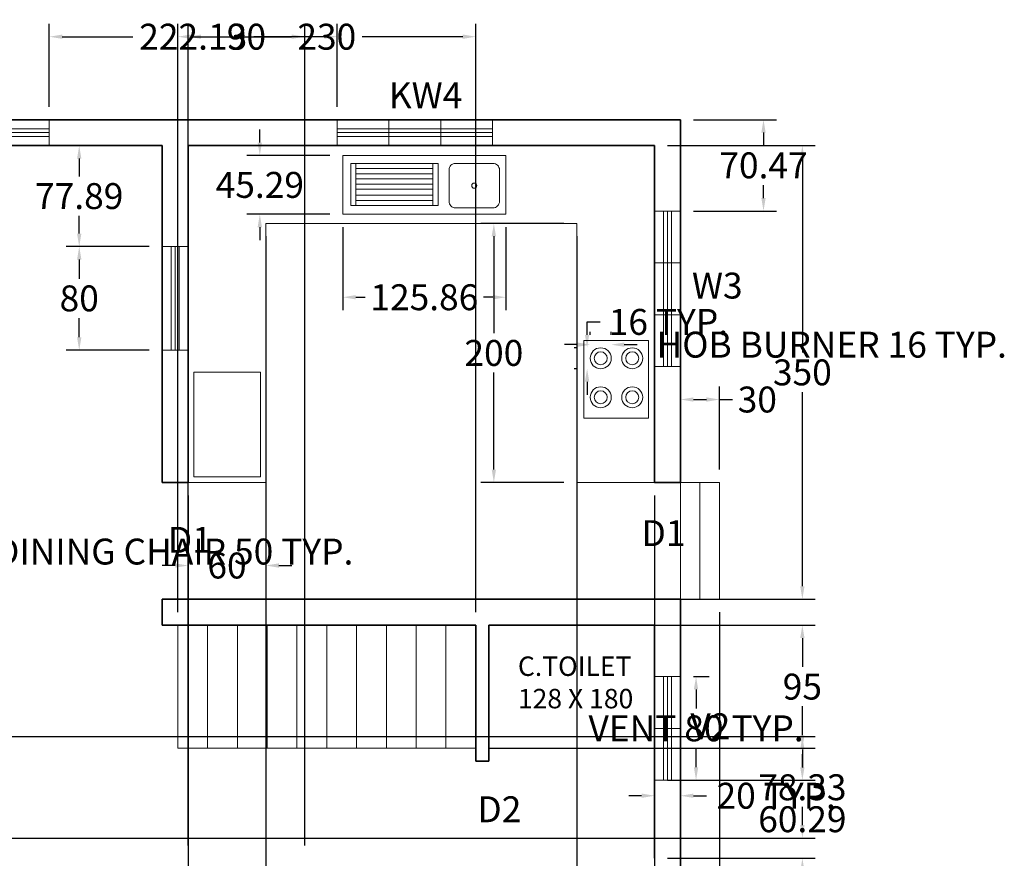
# Model space of a CAD drawing. Units: centimetres. Extents: x 543 to 2148, y 348 to 1642.
# Tile 4 of 4: x 1302 to 2062, y 995 to 1642. Entities that reach past the tile are written whole.
import ezdxf

# ---------------------------------------------------------------- set-up
doc = ezdxf.new("R2010")
doc.units = ezdxf.units.CM
doc.header["$MEASUREMENT"] = 0
for name, color, linetype, lineweight in [('A-ANNO-DIMS', 2, 'Continuous', 18), ('A-ANNO-TEXT', 7, 'Continuous', 18), ('A-AREA-IDEN', 7, 'Continuous', 25), ('A-EQPM', 9, 'Continuous', 18), ('A-FLOR-CASE', 8, 'Continuous', 20), ('A-FLOR-FIXT', 8, 'Continuous', 18), ('A-FLOR-STRS', 7, 'Continuous', 20), ('A-GLAZ', 4, 'Continuous', 18), ('A-WALL', 7, 'Continuous', 35)]:
    doc.layers.add(name, color=color, linetype=linetype, lineweight=lineweight)
doc.styles.get("Standard").update_dxf_attribs({"font": 'arial.ttf'})
doc.dimstyles.get("Standard").update_dxf_attribs({"dimtxt": 20, "dimasz": 10, "dimexe": 10, "dimexo": 10, "dimgap": 5, "dimtad": 0, "dimtih": 1, "dimtoh": 1, "dimdec": 0, "dimzin": 0, "dimdsep": 46, "dimtxsty": 'Standard', "dimcen": 5, "dimadec": 0, "dimazin": 0, "dimtfac": 1, "dimtdec": 0, "dimtofl": 0, "dimtmove": 0, "dimatfit": 3, "dimfxl": 1, "dimtolj": 1, "dimtzin": 0, "dimarcsym": 0})

# ---------------------------------------------------------------- blocks, each defined once
blk = doc.blocks.new('WIN-1200')
for p, q in [((40, 20), (40, 0)), ((80, 20), (80, 0)), ((0, 13), (120, 13)), ((0, 10), (120, 10)), ((0, 7), (120, 7))]:
    blk.add_line(p, q)
blk.add_lwpolyline([(0, 20), (120, 20), (120, 0), (0, 0)], close=True)
blk = doc.blocks.new('VENT-800')
for p, q in [((7, 80), (7, 0)), ((10, 80), (10, 0)), ((13, 80), (13, 0)), ((20, 40), (0, 40)), ((20, 0), (0, 0))]:
    blk.add_line(p, q)
blk.add_lwpolyline([(0, 0), (0, 80), (20, 80), (20, 0)])
blk = doc.blocks.new('HOB-BURNER')
for radius in [8.09, 5]:
    blk.add_circle((8.09, 8.09), radius)
blk = doc.blocks.new('*D15')
at = {"layer": 'A-ANNO-DIMS', "color": 0, "lineweight": -2, "transparency": 16777216}
for p, q in [((1218.09, 1231.81), (1248.09, 1231.81)), ((1258.09, 1231.81), (1268.09, 1231.81)), ((1208.09, 1229.31), (1208.09, 1221.81)), ((1258.09, 1229.31), (1258.09, 1221.81))]:
    blk.add_line(p, q, dxfattribs=at)
at = {"layer": 'A-ANNO-DIMS', "color": 0, "transparency": 16777216}
for points in [[(1218.09, 1233.48), (1218.09, 1230.15), (1208.09, 1231.81)], [(1248.09, 1233.48), (1248.09, 1230.15), (1258.09, 1231.81)]]:
    blk.add_solid(points, dxfattribs=at)
at = {"layer": 'Defpoints', "color": 0, "transparency": 16777216}
for p in [(1208.09, 1239.31), (1258.09, 1239.31), (1258.09, 1231.81)]:
    blk.add_point(p, dxfattribs=at)
at = {"layer": 'A-ANNO-DIMS', "color": 0, "transparency": 16777216, "insert": (1421.4, 1231.81), "char_height": 20, "attachment_point": 5}
blk.add_mtext('\\A1;DINING CHAIR 50 TYP.', dxfattribs=at)
blk = doc.blocks.new('*D17')
at = {"layer": 'A-ANNO-DIMS', "color": 0, "lineweight": -2, "transparency": 16777216}
for p, q in [((1305.14, 955.09), (1305.14, 965.09)), ((1305.14, 965.09), (1315.14, 965.09)), ((1312.14, 945.09), (1315.14, 945.09)), ((1312.14, 925.09), (1315.14, 925.09)), ((1305.14, 915.09), (1305.14, 905.09))]:
    blk.add_line(p, q, dxfattribs=at)
at = {"layer": 'A-ANNO-DIMS', "color": 0, "transparency": 16777216}
for points in [[(1303.47, 955.09), (1306.81, 955.09), (1305.14, 945.09)], [(1303.47, 915.09), (1306.81, 915.09), (1305.14, 925.09)]]:
    blk.add_solid(points, dxfattribs=at)
at = {"layer": 'Defpoints', "color": 0, "transparency": 16777216}
for p in [(1302.14, 945.09), (1305.14, 945.09), (1302.14, 925.09)]:
    blk.add_point(p, dxfattribs=at)
at = {"layer": 'A-ANNO-DIMS', "color": 0, "transparency": 16777216, "insert": (1472.79, 965.09), "char_height": 20, "attachment_point": 5}
blk.add_mtext('\\A1;SCREEN POST 20 TYP.', dxfattribs=at)
blk = doc.blocks.new('*D19')
at = {"layer": 'A-ANNO-DIMS', "color": 0, "lineweight": -2, "transparency": 16777216}
for p, q in [((1742.49, 1399.05), (1742.49, 1401.48)), ((1758.67, 1399.05), (1758.67, 1401.48)), ((1732.49, 1391.48), (1722.49, 1391.48)), ((1768.67, 1391.48), (1778.67, 1391.48))]:
    blk.add_line(p, q, dxfattribs=at)
at = {"layer": 'A-ANNO-DIMS', "color": 0, "transparency": 16777216}
for points in [[(1732.49, 1393.15), (1732.49, 1389.82), (1742.49, 1391.48)], [(1768.67, 1393.15), (1768.67, 1389.82), (1758.67, 1391.48)]]:
    blk.add_solid(points, dxfattribs=at)
at = {"layer": 'Defpoints', "color": 0, "transparency": 16777216}
for p in [(1758.67, 1391.48), (1742.49, 1389.05), (1758.67, 1389.05)]:
    blk.add_point(p, dxfattribs=at)
at = {"layer": 'A-ANNO-DIMS', "color": 0, "transparency": 16777216, "insert": (1928.84, 1391.48), "char_height": 20, "attachment_point": 5}
blk.add_mtext('\\A1;HOB BURNER 16 TYP.', dxfattribs=at)
blk = doc.blocks.new('*D20')
at = {"layer": 'A-ANNO-DIMS', "color": 0, "lineweight": -2, "transparency": 16777216}
for p, q in [((1740.06, 1399.05), (1740.06, 1409.05)), ((1740.06, 1409.05), (1750.06, 1409.05)), ((1732.49, 1389.05), (1730.06, 1389.05)), ((1732.49, 1372.87), (1730.06, 1372.87)), ((1740.06, 1362.87), (1740.06, 1352.87))]:
    blk.add_line(p, q, dxfattribs=at)
at = {"layer": 'A-ANNO-DIMS', "color": 0, "transparency": 16777216}
for points in [[(1738.39, 1399.05), (1741.73, 1399.05), (1740.06, 1389.05)], [(1738.39, 1362.87), (1741.73, 1362.87), (1740.06, 1372.87)]]:
    blk.add_solid(points, dxfattribs=at)
at = {"layer": 'Defpoints', "color": 0, "transparency": 16777216}
for p in [(1740.06, 1389.05), (1742.49, 1389.05), (1742.49, 1372.87)]:
    blk.add_point(p, dxfattribs=at)
at = {"layer": 'A-ANNO-DIMS', "color": 0, "transparency": 16777216, "insert": (1802.79, 1409.05), "char_height": 20, "attachment_point": 5}
blk.add_mtext('\\A1;16 TYP.', dxfattribs=at)
blk = doc.blocks.new('*D27')
at = {"layer": 'A-ANNO-DIMS', "color": 0, "lineweight": -2, "transparency": 16777216}
for p, q in [((1822.14, 1135.38), (1834.14, 1135.38)), ((1824.14, 1125.38), (1824.14, 1110.59)), ((1824.14, 1065.38), (1824.14, 1080.17)), ((1822.14, 1055.38), (1834.14, 1055.38))]:
    blk.add_line(p, q, dxfattribs=at)
at = {"layer": 'A-ANNO-DIMS', "color": 0, "transparency": 16777216}
for points in [[(1822.47, 1125.38), (1825.81, 1125.38), (1824.14, 1135.38)], [(1822.47, 1065.38), (1825.81, 1065.38), (1824.14, 1055.38)]]:
    blk.add_solid(points, dxfattribs=at)
at = {"layer": 'Defpoints', "color": 0, "transparency": 16777216}
for p in [(1812.14, 1135.38), (1824.14, 1135.38), (1812.14, 1055.38)]:
    blk.add_point(p, dxfattribs=at)
at = {"layer": 'A-ANNO-DIMS', "color": 0, "transparency": 16777216, "insert": (1824.14, 1095.38), "char_height": 20, "attachment_point": 5}
blk.add_mtext('\\A1;VENT 80 TYP.', dxfattribs=at)
blk = doc.blocks.new('*D28')
at = {"layer": 'A-ANNO-DIMS', "color": 0, "lineweight": -2, "transparency": 16777216}
for p, q in [((1782.14, 1043.38), (1772.14, 1043.38)), ((1792.14, 1045.38), (1792.14, 1033.38)), ((1812.14, 1045.38), (1812.14, 1033.38)), ((1822.14, 1043.38), (1832.14, 1043.38))]:
    blk.add_line(p, q, dxfattribs=at)
at = {"layer": 'A-ANNO-DIMS', "color": 0, "transparency": 16777216}
for points in [[(1782.14, 1045.05), (1782.14, 1041.72), (1792.14, 1043.38)], [(1822.14, 1045.05), (1822.14, 1041.72), (1812.14, 1043.38)]]:
    blk.add_solid(points, dxfattribs=at)
at = {"layer": 'Defpoints', "color": 0, "transparency": 16777216}
for p in [(1792.14, 1055.38), (1812.14, 1055.38), (1812.14, 1043.38)]:
    blk.add_point(p, dxfattribs=at)
at = {"layer": 'A-ANNO-DIMS', "color": 0, "transparency": 16777216, "insert": (1885.99, 1043.38), "char_height": 20, "attachment_point": 5}
blk.add_mtext('\\A1;20 TYP.', dxfattribs=at)
blk = doc.blocks.new('*D38')
at = {"layer": 'A-ANNO-DIMS', "color": 0, "lineweight": -2, "transparency": 16777216}
for p, q in [((1812.14, 1295.09), (1812.14, 1359.14)), ((1842.14, 1295.09), (1842.14, 1359.14)), ((1822.14, 1349.14), (1832.14, 1349.14)), ((1842.14, 1349.14), (1852.14, 1349.14))]:
    blk.add_line(p, q, dxfattribs=at)
at = {"layer": 'A-ANNO-DIMS', "color": 0, "transparency": 16777216}
for points in [[(1822.14, 1350.81), (1822.14, 1347.48), (1812.14, 1349.14)], [(1832.14, 1350.81), (1832.14, 1347.48), (1842.14, 1349.14)]]:
    blk.add_solid(points, dxfattribs=at)
at = {"layer": 'Defpoints', "color": 0, "transparency": 16777216}
for p in [(1842.14, 1349.14), (1812.14, 1285.09), (1842.14, 1285.09)]:
    blk.add_point(p, dxfattribs=at)
at = {"layer": 'A-ANNO-DIMS', "color": 0, "transparency": 16777216, "insert": (1871.42, 1349.14), "char_height": 20, "attachment_point": 5}
blk.add_mtext('\\A1;30', dxfattribs=at)
blk = doc.blocks.new('*D39')
at = {"layer": 'A-ANNO-DIMS', "color": 0, "lineweight": -2, "transparency": 16777216}
for p, q in [((1432.14, 1275.09), (1432.14, 351.04)), ((1792.14, 1275.09), (1792.14, 351.04)), ((1442.14, 361.04), (1585.09, 361.04)), ((1782.14, 361.04), (1639.19, 361.04))]:
    blk.add_line(p, q, dxfattribs=at)
at = {"layer": 'A-ANNO-DIMS', "color": 0, "transparency": 16777216}
for points in [[(1442.14, 362.71), (1442.14, 359.38), (1432.14, 361.04)], [(1782.14, 362.71), (1782.14, 359.38), (1792.14, 361.04)]]:
    blk.add_solid(points, dxfattribs=at)
at = {"layer": 'Defpoints', "color": 0, "transparency": 16777216}
for p in [(1432.14, 1285.09), (1792.14, 1285.09), (1792.14, 361.04)]:
    blk.add_point(p, dxfattribs=at)
at = {"layer": 'A-ANNO-DIMS', "color": 0, "transparency": 16777216, "insert": (1612.14, 361.04), "char_height": 20, "attachment_point": 5}
blk.add_mtext('\\A1;360', dxfattribs=at)
blk = doc.blocks.new('*D40')
at = {"layer": 'A-ANNO-DIMS', "color": 0, "lineweight": -2, "transparency": 16777216}
for p, q in [((1802.14, 1545.09), (1916.19, 1545.09)), ((1906.19, 1535.09), (1906.19, 1385.31)), ((1906.19, 1205.09), (1906.19, 1354.87)), ((1802.14, 1195.09), (1916.19, 1195.09))]:
    blk.add_line(p, q, dxfattribs=at)
at = {"layer": 'A-ANNO-DIMS', "color": 0, "transparency": 16777216}
for points in [[(1904.52, 1535.09), (1907.86, 1535.09), (1906.19, 1545.09)], [(1904.52, 1205.09), (1907.86, 1205.09), (1906.19, 1195.09)]]:
    blk.add_solid(points, dxfattribs=at)
at = {"layer": 'Defpoints', "color": 0, "transparency": 16777216}
for p in [(1792.14, 1545.09), (1906.19, 1545.09), (1792.14, 1195.09)]:
    blk.add_point(p, dxfattribs=at)
at = {"layer": 'A-ANNO-DIMS', "color": 0, "transparency": 16777216, "insert": (1906.19, 1370.09), "char_height": 20, "attachment_point": 5}
blk.add_mtext('\\A1;350', dxfattribs=at)
blk = doc.blocks.new('*D41')
at = {"layer": 'A-ANNO-DIMS', "color": 0, "lineweight": -2, "transparency": 16777216}
for p, q in [((1424.14, 1185.09), (1424.14, 1639.14)), ((1654.14, 1185.09), (1654.14, 1639.14)), ((1434.14, 1629.14), (1511.91, 1629.14)), ((1644.14, 1629.14), (1566.37, 1629.14))]:
    blk.add_line(p, q, dxfattribs=at)
at = {"layer": 'A-ANNO-DIMS', "color": 0, "transparency": 16777216}
for points in [[(1434.14, 1630.81), (1434.14, 1627.48), (1424.14, 1629.14)], [(1644.14, 1630.81), (1644.14, 1627.48), (1654.14, 1629.14)]]:
    blk.add_solid(points, dxfattribs=at)
at = {"layer": 'Defpoints', "color": 0, "transparency": 16777216}
for p in [(1654.14, 1629.14), (1424.14, 1175.09), (1654.14, 1175.09)]:
    blk.add_point(p, dxfattribs=at)
at = {"layer": 'A-ANNO-DIMS', "color": 0, "transparency": 16777216, "insert": (1539.14, 1629.14), "char_height": 20, "attachment_point": 5}
blk.add_mtext('\\A1;230', dxfattribs=at)
blk = doc.blocks.new('*D42')
at = {"layer": 'A-ANNO-DIMS', "color": 0, "lineweight": -2, "transparency": 16777216}
for p, q in [((1664.14, 1175.09), (1916.19, 1175.09)), ((1906.19, 1165.09), (1906.19, 1142.8)), ((1906.19, 1090.09), (1906.19, 1112.38)), ((1664.14, 1080.09), (1916.19, 1080.09))]:
    blk.add_line(p, q, dxfattribs=at)
at = {"layer": 'A-ANNO-DIMS', "color": 0, "transparency": 16777216}
for points in [[(1904.52, 1165.09), (1907.86, 1165.09), (1906.19, 1175.09)], [(1904.52, 1090.09), (1907.86, 1090.09), (1906.19, 1080.09)]]:
    blk.add_solid(points, dxfattribs=at)
at = {"layer": 'Defpoints', "color": 0, "transparency": 16777216}
for p in [(1654.14, 1175.09), (1906.19, 1175.09), (1654.14, 1080.09)]:
    blk.add_point(p, dxfattribs=at)
at = {"layer": 'A-ANNO-DIMS', "color": 0, "transparency": 16777216, "insert": (1906.19, 1127.59), "char_height": 20, "attachment_point": 5}
blk.add_mtext('\\A1;95', dxfattribs=at)
blk = doc.blocks.new('*D43')
at = {"layer": 'A-ANNO-DIMS', "color": 0, "lineweight": -2, "transparency": 16777216}
for p, q in [((1432.14, 1005.09), (1432.14, 1639.14)), ((1522.14, 1005.09), (1522.14, 1639.14)), ((1442.14, 1629.14), (1457.85, 1629.14)), ((1512.14, 1629.14), (1496.43, 1629.14))]:
    blk.add_line(p, q, dxfattribs=at)
at = {"layer": 'A-ANNO-DIMS', "color": 0, "transparency": 16777216}
for points in [[(1442.14, 1630.81), (1442.14, 1627.48), (1432.14, 1629.14)], [(1512.14, 1630.81), (1512.14, 1627.48), (1522.14, 1629.14)]]:
    blk.add_solid(points, dxfattribs=at)
at = {"layer": 'Defpoints', "color": 0, "transparency": 16777216}
for p in [(1522.14, 1629.14), (1432.14, 995.09), (1522.14, 995.09)]:
    blk.add_point(p, dxfattribs=at)
at = {"layer": 'A-ANNO-DIMS', "color": 0, "transparency": 16777216, "insert": (1477.14, 1629.14), "char_height": 20, "attachment_point": 5}
blk.add_mtext('\\A1;90', dxfattribs=at)
blk = doc.blocks.new('*D50')
at = {"layer": 'A-ANNO-DIMS', "color": 0, "lineweight": -2, "transparency": 16777216}
for p, q in [((1325.01, 1575.09), (1325.01, 1639.14)), ((1547.14, 1575.09), (1547.14, 1639.14)), ((1335.01, 1629.14), (1389.39, 1629.14)), ((1537.14, 1629.14), (1482.76, 1629.14))]:
    blk.add_line(p, q, dxfattribs=at)
at = {"layer": 'A-ANNO-DIMS', "color": 0, "transparency": 16777216}
for points in [[(1335.01, 1630.81), (1335.01, 1627.48), (1325.01, 1629.14)], [(1537.14, 1630.81), (1537.14, 1627.48), (1547.14, 1629.14)]]:
    blk.add_solid(points, dxfattribs=at)
at = {"layer": 'Defpoints', "color": 0, "transparency": 16777216}
for p in [(1547.14, 1629.14), (1325.01, 1565.09), (1547.14, 1565.09)]:
    blk.add_point(p, dxfattribs=at)
at = {"layer": 'A-ANNO-DIMS', "color": 0, "transparency": 16777216, "insert": (1436.07, 1629.14), "char_height": 20, "attachment_point": 5}
blk.add_mtext('\\A1;222.13', dxfattribs=at)
blk = doc.blocks.new('*D51')
at = {"layer": 'A-ANNO-DIMS', "color": 0, "lineweight": -2, "transparency": 16777216}
for p, q in [((1822.14, 1565.09), (1886.19, 1565.09)), ((1876.19, 1555.09), (1876.19, 1545.07)), ((1876.19, 1504.62), (1876.19, 1514.64)), ((1822.14, 1494.62), (1886.19, 1494.62))]:
    blk.add_line(p, q, dxfattribs=at)
at = {"layer": 'A-ANNO-DIMS', "color": 0, "transparency": 16777216}
for points in [[(1874.52, 1555.09), (1877.86, 1555.09), (1876.19, 1565.09)], [(1874.52, 1504.62), (1877.86, 1504.62), (1876.19, 1494.62)]]:
    blk.add_solid(points, dxfattribs=at)
at = {"layer": 'Defpoints', "color": 0, "transparency": 16777216}
for p in [(1812.14, 1565.09), (1812.14, 1494.62), (1876.19, 1494.62)]:
    blk.add_point(p, dxfattribs=at)
at = {"layer": 'A-ANNO-DIMS', "color": 0, "transparency": 16777216, "insert": (1876.19, 1529.85), "char_height": 20, "attachment_point": 5}
blk.add_mtext('\\A1;70.47', dxfattribs=at)
blk = doc.blocks.new('*D52')
at = {"layer": 'A-ANNO-DIMS', "color": 0, "lineweight": -2, "transparency": 16777216}
for p, q in [((1906.19, 1065.38), (1906.19, 1075.38)), ((1802.14, 1055.38), (1916.19, 1055.38)), ((1802.14, 995.09), (1916.19, 995.09)), ((1906.19, 985.09), (1906.19, 975.09))]:
    blk.add_line(p, q, dxfattribs=at)
at = {"layer": 'A-ANNO-DIMS', "color": 0, "transparency": 16777216}
for points in [[(1904.52, 1065.38), (1907.86, 1065.38), (1906.19, 1055.38)], [(1904.52, 985.09), (1907.86, 985.09), (1906.19, 995.09)]]:
    blk.add_solid(points, dxfattribs=at)
at = {"layer": 'Defpoints', "color": 0, "transparency": 16777216}
for p in [(1792.14, 1055.38), (1906.19, 1055.38), (1792.14, 995.09)]:
    blk.add_point(p, dxfattribs=at)
at = {"layer": 'A-ANNO-DIMS', "color": 0, "transparency": 16777216, "insert": (1906.19, 1025.24), "char_height": 20, "attachment_point": 5}
blk.add_mtext('\\A1;60.29', dxfattribs=at)
blk = doc.blocks.new('*D59')
at = {"layer": 'A-ANNO-DIMS', "color": 0, "lineweight": -2, "transparency": 16777216}
for p, q in [((717.14, 1089.08), (1916.19, 1089.08)), ((1906.19, 1079.08), (1906.19, 1065.14)), ((1906.19, 1020.76), (1906.19, 1034.7)), ((717.14, 1010.76), (1916.19, 1010.76))]:
    blk.add_line(p, q, dxfattribs=at)
at = {"layer": 'A-ANNO-DIMS', "color": 0, "transparency": 16777216}
for points in [[(1904.52, 1079.08), (1907.86, 1079.08), (1906.19, 1089.08)], [(1904.52, 1020.76), (1907.86, 1020.76), (1906.19, 1010.76)]]:
    blk.add_solid(points, dxfattribs=at)
at = {"layer": 'Defpoints', "color": 0, "transparency": 16777216}
for p in [(707.14, 1089.08), (1906.19, 1089.08), (707.14, 1010.76)]:
    blk.add_point(p, dxfattribs=at)
at = {"layer": 'A-ANNO-DIMS', "color": 0, "transparency": 16777216, "insert": (1906.19, 1049.92), "char_height": 20, "attachment_point": 5}
blk.add_mtext('\\A1;78.33', dxfattribs=at)
blk = doc.blocks.new('*D61')
at = {"layer": 'A-ANNO-DIMS', "color": 0, "lineweight": -2, "transparency": 16777216}
for p, q in [((1492.14, 1475.09), (1492.14, 351.04)), ((1732.14, 1475.09), (1732.14, 351.04)), ((1502.14, 361.04), (1584.91, 361.04)), ((1722.14, 361.04), (1639.37, 361.04))]:
    blk.add_line(p, q, dxfattribs=at)
at = {"layer": 'A-ANNO-DIMS', "color": 0, "transparency": 16777216}
for points in [[(1502.14, 362.71), (1502.14, 359.38), (1492.14, 361.04)], [(1722.14, 362.71), (1722.14, 359.38), (1732.14, 361.04)]]:
    blk.add_solid(points, dxfattribs=at)
at = {"layer": 'Defpoints', "color": 0, "transparency": 16777216}
for p in [(1492.14, 1485.09), (1732.14, 1485.09), (1732.14, 361.04)]:
    blk.add_point(p, dxfattribs=at)
at = {"layer": 'A-ANNO-DIMS', "color": 0, "transparency": 16777216, "insert": (1612.14, 361.04), "char_height": 20, "attachment_point": 5}
blk.add_mtext('\\A1;240', dxfattribs=at)
blk = doc.blocks.new('*D62')
at = {"layer": 'A-ANNO-DIMS', "color": 0, "lineweight": -2, "transparency": 16777216}
for p, q in [((1722.14, 1485.09), (1658.09, 1485.09)), ((1668.09, 1475.09), (1668.09, 1400.3)), ((1668.09, 1295.09), (1668.09, 1369.88)), ((1722.14, 1285.09), (1658.09, 1285.09))]:
    blk.add_line(p, q, dxfattribs=at)
at = {"layer": 'A-ANNO-DIMS', "color": 0, "transparency": 16777216}
for points in [[(1666.42, 1475.09), (1669.76, 1475.09), (1668.09, 1485.09)], [(1666.42, 1295.09), (1669.76, 1295.09), (1668.09, 1285.09)]]:
    blk.add_solid(points, dxfattribs=at)
at = {"layer": 'Defpoints', "color": 0, "transparency": 16777216}
for p in [(1668.09, 1485.09), (1732.14, 1485.09), (1732.14, 1285.09)]:
    blk.add_point(p, dxfattribs=at)
at = {"layer": 'A-ANNO-DIMS', "color": 0, "transparency": 16777216, "insert": (1668.09, 1385.09), "char_height": 20, "attachment_point": 5}
blk.add_mtext('\\A1;200', dxfattribs=at)
blk = doc.blocks.new('*D63')
at = {"layer": 'A-ANNO-DIMS', "color": 0, "lineweight": -2, "transparency": 16777216}
for p, q in [((1432.14, 1275.09), (1432.14, 1211.04)), ((1492.14, 1275.09), (1492.14, 1211.04)), ((1422.14, 1221.04), (1412.14, 1221.04)), ((1502.14, 1221.04), (1512.14, 1221.04))]:
    blk.add_line(p, q, dxfattribs=at)
at = {"layer": 'A-ANNO-DIMS', "color": 0, "transparency": 16777216}
for points in [[(1422.14, 1222.71), (1422.14, 1219.38), (1432.14, 1221.04)], [(1502.14, 1222.71), (1502.14, 1219.38), (1492.14, 1221.04)]]:
    blk.add_solid(points, dxfattribs=at)
at = {"layer": 'Defpoints', "color": 0, "transparency": 16777216}
for p in [(1432.14, 1285.09), (1492.14, 1285.09), (1432.14, 1221.04)]:
    blk.add_point(p, dxfattribs=at)
at = {"layer": 'A-ANNO-DIMS', "color": 0, "transparency": 16777216, "insert": (1462.14, 1221.04), "char_height": 20, "attachment_point": 5}
blk.add_mtext('\\A1;60', dxfattribs=at)
blk = doc.blocks.new('*D68')
at = {"layer": 'A-ANNO-DIMS', "color": 0, "lineweight": -2, "transparency": 16777216}
for p, q in [((1842.14, 1185.09), (1842.14, 351.04)), ((637.14, 415.09), (637.14, 351.04)), ((647.14, 361.04), (1205.64, 361.04)), ((1832.14, 361.04), (1273.64, 361.04))]:
    blk.add_line(p, q, dxfattribs=at)
at = {"layer": 'A-ANNO-DIMS', "color": 0, "transparency": 16777216}
for points in [[(647.14, 362.71), (647.14, 359.38), (637.14, 361.04)], [(1832.14, 362.71), (1832.14, 359.38), (1842.14, 361.04)]]:
    blk.add_solid(points, dxfattribs=at)
at = {"layer": 'Defpoints', "color": 0, "transparency": 16777216}
for p in [(1842.14, 1195.09), (637.14, 425.09), (1842.14, 361.04)]:
    blk.add_point(p, dxfattribs=at)
at = {"layer": 'A-ANNO-DIMS', "color": 0, "transparency": 16777216, "insert": (1239.64, 361.04), "char_height": 20, "attachment_point": 5}
blk.add_mtext('\\A1;1205', dxfattribs=at)
blk = doc.blocks.new('*D69')
at = {"layer": 'A-ANNO-DIMS', "color": 0, "lineweight": -2, "transparency": 16777216}
for p, q in [((1551.51, 1482.13), (1551.51, 1418.08)), ((1677.37, 1482.13), (1677.37, 1418.08)), ((1561.51, 1428.08), (1568.87, 1428.08)), ((1667.37, 1428.08), (1660, 1428.08))]:
    blk.add_line(p, q, dxfattribs=at)
at = {"layer": 'A-ANNO-DIMS', "color": 0, "transparency": 16777216}
for points in [[(1561.51, 1429.74), (1561.51, 1426.41), (1551.51, 1428.08)], [(1667.37, 1429.74), (1667.37, 1426.41), (1677.37, 1428.08)]]:
    blk.add_solid(points, dxfattribs=at)
at = {"layer": 'Defpoints', "color": 0, "transparency": 16777216}
for p in [(1551.51, 1492.13), (1677.37, 1492.13), (1551.51, 1428.08)]:
    blk.add_point(p, dxfattribs=at)
at = {"layer": 'A-ANNO-DIMS', "color": 0, "transparency": 16777216, "insert": (1614.44, 1428.08), "char_height": 20, "attachment_point": 5}
blk.add_mtext('\\A1;125.86', dxfattribs=at)
blk = doc.blocks.new('*D70')
at = {"layer": 'A-ANNO-DIMS', "color": 0, "lineweight": -2, "transparency": 16777216}
for p, q in [((1487.46, 1547.42), (1487.46, 1557.42)), ((1541.51, 1537.42), (1477.46, 1537.42)), ((1541.51, 1492.13), (1477.46, 1492.13)), ((1487.46, 1482.13), (1487.46, 1472.13))]:
    blk.add_line(p, q, dxfattribs=at)
at = {"layer": 'A-ANNO-DIMS', "color": 0, "transparency": 16777216}
for points in [[(1485.79, 1547.42), (1489.13, 1547.42), (1487.46, 1537.42)], [(1485.79, 1482.13), (1489.13, 1482.13), (1487.46, 1492.13)]]:
    blk.add_solid(points, dxfattribs=at)
at = {"layer": 'Defpoints', "color": 0, "transparency": 16777216}
for p in [(1487.46, 1537.42), (1551.51, 1537.42), (1551.51, 1492.13)]:
    blk.add_point(p, dxfattribs=at)
at = {"layer": 'A-ANNO-DIMS', "color": 0, "transparency": 16777216, "insert": (1487.46, 1514.77), "char_height": 20, "attachment_point": 5}
blk.add_mtext('\\A1;45.29', dxfattribs=at)
blk = doc.blocks.new('*D71')
at = {"layer": 'A-ANNO-DIMS', "color": 0, "lineweight": -2, "transparency": 16777216}
for p, q in [((1402.14, 1467.2), (1338.09, 1467.2)), ((1348.09, 1457.2), (1348.09, 1442.41)), ((1348.09, 1397.2), (1348.09, 1411.99)), ((1402.14, 1387.2), (1338.09, 1387.2))]:
    blk.add_line(p, q, dxfattribs=at)
at = {"layer": 'A-ANNO-DIMS', "color": 0, "transparency": 16777216}
for points in [[(1346.42, 1457.2), (1349.76, 1457.2), (1348.09, 1467.2)], [(1346.42, 1397.2), (1349.76, 1397.2), (1348.09, 1387.2)]]:
    blk.add_solid(points, dxfattribs=at)
at = {"layer": 'Defpoints', "color": 0, "transparency": 16777216}
for p in [(1348.09, 1467.2), (1412.14, 1467.2), (1412.14, 1387.2)]:
    blk.add_point(p, dxfattribs=at)
at = {"layer": 'A-ANNO-DIMS', "color": 0, "transparency": 16777216, "insert": (1348.09, 1427.2), "char_height": 20, "attachment_point": 5}
blk.add_mtext('\\A1;80', dxfattribs=at)
blk = doc.blocks.new('*D72')
at = {"layer": 'A-ANNO-DIMS', "color": 0, "lineweight": -2, "transparency": 16777216}
for p, q in [((1402.14, 1545.09), (1338.09, 1545.09)), ((1348.09, 1535.09), (1348.09, 1521.36)), ((1348.09, 1477.2), (1348.09, 1490.94)), ((1402.14, 1467.2), (1338.09, 1467.2))]:
    blk.add_line(p, q, dxfattribs=at)
at = {"layer": 'A-ANNO-DIMS', "color": 0, "transparency": 16777216}
for points in [[(1346.42, 1535.09), (1349.76, 1535.09), (1348.09, 1545.09)], [(1346.42, 1477.2), (1349.76, 1477.2), (1348.09, 1467.2)]]:
    blk.add_solid(points, dxfattribs=at)
at = {"layer": 'Defpoints', "color": 0, "transparency": 16777216}
for p in [(1348.09, 1545.09), (1412.14, 1545.09), (1412.14, 1467.2)]:
    blk.add_point(p, dxfattribs=at)
at = {"layer": 'A-ANNO-DIMS', "color": 0, "transparency": 16777216, "insert": (1348.09, 1506.15), "char_height": 20, "attachment_point": 5}
blk.add_mtext('\\A1;77.89', dxfattribs=at)

msp = doc.modelspace()

# ---------------------------------------------------------------- linework, layer by layer
at = {"layer": 'A-EQPM'}
for points in [[(1737.54, 1394.631), (1787.54, 1394.631), (1787.54, 1334.631), (1737.54, 1334.631)], [(1436.469, 1370.378), (1487.939, 1370.378), (1487.939, 1289.609), (1436.469, 1289.609)]]:
    msp.add_lwpolyline(points, close=True, dxfattribs=at)
at = {"layer": 'A-FLOR-CASE'}
for p, q in [((1492.141, 1285.092), (1492.141, 1485.092)), ((1492.141, 1485.092), (1732.141, 1485.092)), ((1732.141, 1485.092), (1732.141, 1285.092)), ((1432.141, 1285.092), (1492.141, 1285.092)), ((1732.141, 1285.092), (1792.141, 1285.092))]:
    msp.add_line(p, q, dxfattribs=at)
at = {"layer": 'A-FLOR-FIXT'}
for p, q in [((1561.615, 1531.348), (1561.615, 1498.848)), ((1621.042, 1498.848), (1621.042, 1531.348)), ((1621.042, 1527.357), (1561.615, 1527.357)), ((1621.042, 1523.357), (1561.615, 1523.357)), ((1621.042, 1519.357), (1561.615, 1519.357)), ((1621.042, 1515.357), (1561.615, 1515.357)), ((1621.042, 1511.357), (1561.615, 1511.357)), ((1561.615, 1506.839), (1621.042, 1506.839)), ((1561.615, 1502.839), (1621.042, 1502.839))]:
    msp.add_line(p, q, dxfattribs=at)
for points in [[(1551.509, 1537.416), (1677.365, 1537.416), (1677.365, 1492.128), (1551.509, 1492.128)], [(1625.034, 1531.348), (1557.624, 1531.348), (1557.624, 1498.848), (1625.034, 1498.848)]]:
    msp.add_lwpolyline(points, close=True, dxfattribs=at)
msp.add_lwpolyline([(1667.415, 1531.348), (1638.517, 1531.348, 0.4142136), (1633.517, 1526.348), (1633.517, 1502.075, 0.4142136), (1638.517, 1497.075), (1667.415, 1497.075, 0.4142136), (1672.415, 1502.075), (1672.415, 1526.348, 0.4142136)], format="xyb", close=True, dxfattribs=at)
msp.add_circle((1652.966, 1514.211), 2, dxfattribs=at)
at = {"layer": 'A-FLOR-STRS'}
for p, q in [((1812.141, 1285.092), (1842.141, 1285.092)), ((1812.141, 1285.092), (1812.141, 1195.092)), ((1827.141, 1285.092), (1827.141, 1195.092)), ((1842.141, 1285.092), (1842.141, 1195.092)), ((1842.141, 1195.092), (1812.141, 1195.092)), ((1424.141, 1175.092), (1424.141, 1080.092)), ((1447.141, 1175.092), (1447.141, 1080.092)), ((1470.141, 1175.092), (1470.141, 1080.092)), ((1493.141, 1175.092), (1493.141, 1080.092)), ((1516.141, 1175.092), (1516.141, 1080.092)), ((1539.141, 1175.092), (1539.141, 1080.092)), ((1562.141, 1175.092), (1562.141, 1080.092)), ((1585.141, 1175.092), (1585.141, 1080.092)), ((1608.141, 1175.092), (1608.141, 1080.092)), ((1631.141, 1175.092), (1631.141, 1080.092)), ((1424.141, 1080.092), (1654.141, 1080.092))]:
    msp.add_line(p, q, dxfattribs=at)
at = {"layer": 'A-GLAZ'}
for p, q in [((1419.141, 1467.202), (1419.141, 1387.202)), ((1422.141, 1467.202), (1422.141, 1387.202)), ((1425.141, 1467.202), (1425.141, 1387.202)), ((1432.141, 1387.202), (1412.141, 1387.202))]:
    msp.add_line(p, q, dxfattribs=at)
msp.add_lwpolyline([(1412.141, 1387.202), (1412.141, 1467.202), (1432.141, 1467.202), (1432.141, 1387.202)], dxfattribs=at)
at = {"layer": 'A-WALL'}
for p, q in [((1412.141, 1565.092), (687.141, 1565.092)), ((1812.141, 1565.092), (1412.141, 1565.092)), ((1812.141, 1285.092), (1812.141, 1565.092)), ((1087.141, 1545.092), (1412.141, 1545.092)), ((1412.141, 1525.092), (1412.141, 1545.092)), ((1412.141, 1545.092), (1412.141, 1285.092)), ((1432.141, 1545.092), (1432.141, 1525.092)), ((1792.141, 1545.092), (1432.141, 1545.092)), ((1432.141, 1545.092), (1432.141, 1285.092)), ((1792.141, 1285.092), (1792.141, 1545.092)), ((1432.141, 1285.092), (1412.141, 1285.092)), ((1812.141, 1285.092), (1792.141, 1285.092)), ((1432.141, 1195.092), (1412.141, 1195.092)), ((1412.141, 1195.092), (1412.141, 1175.092)), ((1432.141, 1195.092), (1792.141, 1195.092)), ((1812.141, 1195.092), (1792.141, 1195.092)), ((1812.141, 635.092), (1812.141, 1195.092)), ((1654.141, 1175.092), (1412.141, 1175.092)), ((1654.141, 1175.092), (1654.141, 1070.092)), ((1792.141, 1175.092), (1664.141, 1175.092)), ((1664.141, 1175.092), (1664.141, 1070.092)), ((1792.141, 995.092), (1792.141, 1175.092)), ((1654.141, 1080.092), (1654.141, 1070.092)), ((1654.141, 1070.092), (1664.141, 1070.092))]:
    msp.add_line(p, q, dxfattribs=at)

# ---------------------------------------------------------------- block references
at = {"layer": 'A-EQPM'}
for p in [(1742.487, 1372.869), (1766.79, 1372.869), (1742.487, 1342.77), (1766.79, 1342.77)]:
    msp.add_blockref('HOB-BURNER', p, dxfattribs=at)
at = {"layer": 'A-GLAZ'}
for name, p in [('WIN-1200', (1205.005, 1545.092)), ('WIN-1200', (1547.138, 1545.092)), ('VENT-800', (1792.141, 1055.382))]:
    msp.add_blockref(name, p, dxfattribs=at)
at = {"layer": 'A-GLAZ', "rotation": 270.0000000000002}
msp.add_blockref('WIN-1200', (1792.141, 1494.618), dxfattribs=at)

# ---------------------------------------------------------------- texts
at = {"layer": 'A-ANNO-TEXT', "char_height": 20, "attachment_point": 1}
for s, insert in [('KW4', (1587.011, 1593.959)), ('W3', (1820.963, 1447.071)), ('D1', (1782.084, 1256.031)), ('D1', (1416.525, 1250.84)), ('V2', (1819.743, 1107.008)), ('D2', (1655.389, 1042.91))]:
    msp.add_mtext_dynamic_manual_height_columns(s, width=246.06417, gutter_width=1, heights=[0], dxfattribs=dict(at, insert=insert))
at = {"layer": 'A-AREA-IDEN', "insert": (1686.645, 1150.838), "char_height": 15, "attachment_point": 1}
msp.add_mtext_dynamic_manual_height_columns('C.TOILET\\P128 X 180', width=246.06417, gutter_width=1, heights=[0], dxfattribs=at)

# ---------------------------------------------------------------- dimensions: what is measured, and where the dimension line sits
at = {"layer": 'A-ANNO-DIMS'}
for base, p1, p2, override, picture, middle in [((1547.138, 1629.142), (1325.005, 1565.092), (1547.138, 1565.092), {"dimdec": 2, "dimlfac": 1, "dimrnd": 0, "dimzin": 0, "dimdsep": 46, "dimlunit": 2}, '*D50', (1436.072, 1629.142)), ((1654.141, 1629.142), (1424.141, 1175.092), (1654.141, 1175.092), {"dimdec": 0, "dimlfac": 1, "dimrnd": 0, "dimzin": 0, "dimdsep": 46, "dimlunit": 2}, '*D41', (1539.141, 1629.142)), ((1522.141, 1629.142), (1432.141, 995.092), (1522.141, 995.092), {"dimdec": 0, "dimlfac": 1, "dimrnd": 0, "dimzin": 0, "dimdsep": 46, "dimlunit": 2}, '*D43', (1477.141, 1629.142)), ((1732.141, 361.042), (1492.141, 1485.092), (1732.141, 1485.092), {"dimdec": 0, "dimlfac": 1, "dimrnd": 0, "dimzin": 0, "dimdsep": 46, "dimlunit": 2}, '*D61', (1612.141, 361.042)), ((1842.141, 1349.142), (1812.141, 1285.092), (1842.141, 1285.092), {"dimdec": 0, "dimlfac": 1, "dimrnd": 0, "dimzin": 0, "dimdsep": 46, "dimlunit": 2}, '*D38', (1871.425, 1349.142)), ((1792.141, 361.042), (1432.141, 1285.092), (1792.141, 1285.092), {"dimdec": 0, "dimlfac": 1, "dimrnd": 0, "dimzin": 0, "dimdsep": 46, "dimlunit": 2}, '*D39', (1612.141, 361.042)), ((1842.141, 361.042), (637.141, 425.092), (1842.141, 1195.092), {"dimdec": 0, "dimlfac": 1, "dimrnd": 0, "dimzin": 0, "dimdsep": 46, "dimlunit": 2}, '*D68', (1239.641, 361.042))]:
    dim = msp.add_linear_dim(base=base, p1=p1, p2=p2, dimstyle='Standard', override=override, dxfattribs=at)
    dim.commit()
    dim.dimension.update_dxf_attribs({"geometry": picture, "text_midpoint": middle})
for base, p1, p2, angle, override, picture, middle in [((1876.191, 1494.618), (1812.141, 1565.092), (1812.141, 1494.618), 270, {"dimdec": 2, "dimlfac": 1, "dimrnd": 0, "dimzin": 0, "dimdsep": 46, "dimlunit": 2}, '*D51', (1876.191, 1529.855)), ((1487.459, 1537.416), (1551.509, 1492.128), (1551.509, 1537.416), 90, {"dimdec": 2, "dimlfac": 1, "dimrnd": 0, "dimzin": 0, "dimdsep": 46, "dimlunit": 2}, '*D70', (1487.459, 1514.772)), ((1348.091, 1545.092), (1412.141, 1467.202), (1412.141, 1545.092), 90, {"dimdec": 2, "dimlfac": 1, "dimrnd": 0, "dimzin": 0, "dimdsep": 46, "dimlunit": 2}, '*D72', (1348.091, 1506.147)), ((1906.191, 1545.092), (1792.141, 1195.092), (1792.141, 1545.092), 90, {"dimdec": 0, "dimlfac": 1, "dimrnd": 0, "dimzin": 0, "dimdsep": 46, "dimlunit": 2}, '*D40', (1906.191, 1370.092)), ((1551.509, 1428.078), (1677.365, 1492.128), (1551.509, 1492.128), 180, {"dimdec": 2, "dimlfac": 1, "dimrnd": 0, "dimzin": 0, "dimdsep": 46, "dimlunit": 2}, '*D69', (1614.437, 1428.078)), ((1668.091, 1485.092), (1732.141, 1285.092), (1732.141, 1485.092), 90, {"dimdec": 0, "dimlfac": 1, "dimrnd": 0, "dimzin": 0, "dimdsep": 46, "dimlunit": 2}, '*D62', (1668.091, 1385.092)), ((1348.091, 1467.202), (1412.141, 1387.202), (1412.141, 1467.202), 90, {"dimdec": 0, "dimlfac": 1, "dimrnd": 0, "dimzin": 0, "dimdsep": 46, "dimlunit": 2}, '*D71', (1348.091, 1427.202)), ((1432.141, 1221.042), (1492.141, 1285.092), (1432.141, 1285.092), 180, {"dimdec": 0, "dimlfac": 1, "dimrnd": 0, "dimzin": 0, "dimdsep": 46, "dimlunit": 2}, '*D63', (1462.141, 1221.042)), ((1906.191, 1175.092), (1654.141, 1080.092), (1654.141, 1175.092), 90, {"dimdec": 0, "dimlfac": 1, "dimrnd": 0, "dimzin": 0, "dimdsep": 46, "dimlunit": 2}, '*D42', (1906.191, 1127.592)), ((1906.1909, 1089.0833), (707.1409, 1010.7581), (707.1409, 1089.0833), 90, {"dimdec": 2, "dimlfac": 1, "dimrnd": 0, "dimzin": 0, "dimdsep": 46, "dimlunit": 2}, '*D59', (1906.1909, 1049.9207)), ((1906.191, 1055.382), (1792.141, 995.092), (1792.141, 1055.382), 90, {"dimdec": 2, "dimlfac": 1, "dimrnd": 0, "dimzin": 0, "dimdsep": 46, "dimlunit": 2}, '*D52', (1906.191, 1025.237))]:
    dim = msp.add_linear_dim(base=base, p1=p1, p2=p2, angle=angle, dimstyle='Standard', override=override, dxfattribs=at)
    dim.commit()
    dim.dimension.update_dxf_attribs({"geometry": picture, "text_midpoint": middle})
for base, p1, p2, text, picture, middle in [((1758.672, 1391.482), (1742.487, 1389.055), (1758.672, 1389.055), 'HOB BURNER <> TYP.', '*D19', (1928.836, 1391.482)), ((1812.141, 1043.382), (1792.141, 1055.382), (1812.141, 1055.382), '<> TYP.', '*D28', (1885.988, 1043.382))]:
    dim = msp.add_linear_dim(base=base, p1=p1, p2=p2, text=text, dimstyle='Standard', override={"dimdec": 0, "dimlfac": 1, "dimrnd": 0, "dimzin": 0, "dimdsep": 46, "dimlunit": 2}, dxfattribs=at)
    dim.commit()
    dim.dimension.update_dxf_attribs({"geometry": picture, "text_midpoint": middle})
for base, p1, p2, angle, text, picture, middle in [((1740.059, 1389.055), (1742.487, 1372.869), (1742.487, 1389.055), 90, '<> TYP.', '*D20', (1802.795, 1409.055)), ((1258.094, 1231.813), (1208.094, 1239.313), (1258.094, 1239.313), 0, 'DINING CHAIR <> TYP.', '*D15', (1421.396, 1231.813)), ((1824.141, 1135.382), (1812.141, 1055.382), (1812.141, 1135.382), 90, 'VENT <> TYP.', '*D27', (1824.141, 1095.382)), ((1305.141, 945.092), (1302.141, 925.092), (1302.141, 945.092), 90, 'SCREEN POST <> TYP.', '*D17', (1472.788, 965.092))]:
    dim = msp.add_linear_dim(base=base, p1=p1, p2=p2, angle=angle, text=text, dimstyle='Standard', override={"dimdec": 0, "dimlfac": 1, "dimrnd": 0, "dimzin": 0, "dimdsep": 46, "dimlunit": 2}, dxfattribs=at)
    dim.commit()
    dim.dimension.update_dxf_attribs({"geometry": picture, "text_midpoint": middle})

doc.saveas('drawing.dxf')
